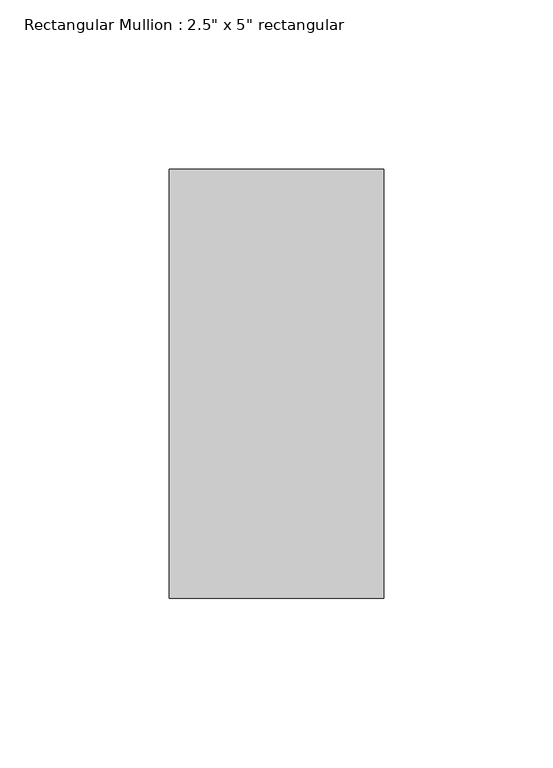
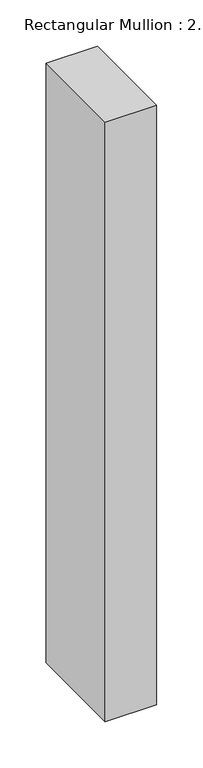
"""IFC4 building model written with IfcOpenShell, lengths in millimetres: member geometry."""

from ifc_helpers import new_model, si_unit, frame, origin, place, context, project, spatial, polyline, outline, extrude, source, transform, mapped, element, save


def member_18a184ad(model_context):
    return source(origin(), model_context, "Body", "SweptSolid", [
        extrude(outline(polyline([(31.75, 63.5), (31.75, -63.5), (-31.75, -63.5), (-31.75, 63.5), (31.75, 63.5)])), frame((0.0, 0.0, -787.4), z_axis=(0.0, 0.0, 1.0), x_axis=(1.0, 0.0, 0.0)), (0.0, 0.0, 1.0), 787.4),
    ])


if __name__ == "__main__":
    model = new_model("IFC4")
    model_context = context("Model", 3, world=origin())
    ifc_project = project(units=[si_unit("LENGTHUNIT", "METRE", prefix="MILLI")], contexts=[model_context])
    site = spatial("IfcSite", under=ifc_project)
    building = spatial("IfcBuilding", under=site)
    placement = place(None, origin())
    member_shape = member_18a184ad(model_context)
    element("IfcMember", 1, ObjectType="Rectangular Mullion : 2.5\" x 5\" rectangular", at=placement, inside=building, context=model_context, shape_type="MappedRepresentation", body=[
        mapped(member_shape, transform((0.0, 0.0, 0.0), x_axis=(1.0, 0.0, 0.0), y_axis=(0.0, 1.0, 0.0), z_axis=(0.0, 0.0, 1.0))),
    ])
    save(model, "model.ifc")

# Revit data of these elements
# Type "Rectangular Mullion : 2.5\" x 5\" rectangular"
#   built-in parameter 1007304 = 0.416667 (stored number, unit not read)
#   built-in parameter 1007301 = 0.104167 (stored number, unit not read)
#   built-in parameter 1007300 = 0.104167 (stored number, unit not read)
# Element 1 (IfcMember, "Rectangular Mullion : 2.5\" x 5\" rectangular")
#   Materials on its faces: "BLACK MATERIAL"
# Materials
#   "BLACK MATERIAL": class "Generic", colour RGB 120 120 120, transparency 0, Cost = 0
